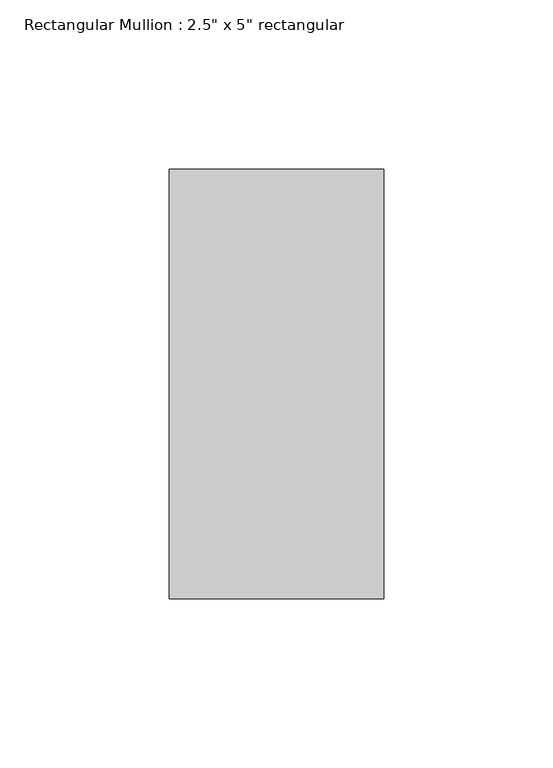
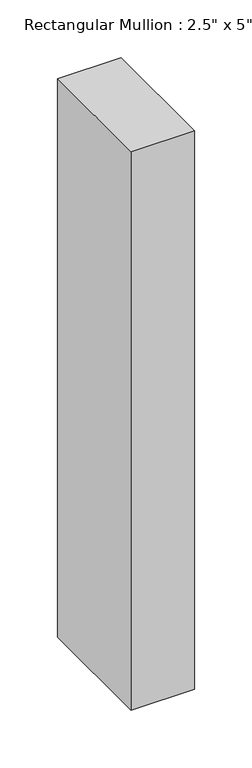
"""IFC4 building model written with IfcOpenShell, lengths in millimetres: member geometry."""

from ifc_helpers import new_model, si_unit, frame, origin, place, context, project, spatial, polyline, outline, extrude, source, transform, mapped, element, save


def member_e5d39754(model_context):
    return source(origin(), model_context, "Body", "SweptSolid", [
        extrude(outline(polyline([(0.0, 63.5), (0.0, -63.5), (-63.5, -63.5), (-63.5, 63.5), (0.0, 63.5)])), frame((0.0, 0.0, -590.55), z_axis=(0.0, 0.0, 1.0), x_axis=(1.0, 0.0, 0.0)), (0.0, 0.0, 1.0), 590.55),
    ])


if __name__ == "__main__":
    model = new_model("IFC4")
    model_context = context("Model", 3, world=origin())
    ifc_project = project(units=[si_unit("LENGTHUNIT", "METRE", prefix="MILLI")], contexts=[model_context])
    site = spatial("IfcSite", under=ifc_project)
    building = spatial("IfcBuilding", under=site)
    placement = place(None, origin())
    member_shape = member_e5d39754(model_context)
    element("IfcMember", 1, ObjectType="Rectangular Mullion : 2.5\" x 5\" rectangular", at=placement, inside=building, context=model_context, shape_type="MappedRepresentation", body=[
        mapped(member_shape, transform((0.0, 0.0, 0.0), x_axis=(1.0, 0.0, 0.0), y_axis=(0.0, 1.0, 0.0), z_axis=(0.0, 0.0, 1.0))),
    ])
    save(model, "model.ifc")

# Revit data of these elements
# Type "Rectangular Mullion : 2.5\" x 5\" rectangular"
#   built-in parameter 1007304 = 0.416667 (stored number, unit not read)
#   built-in parameter 1007301 = 0.104167 (stored number, unit not read)
#   built-in parameter 1007300 = 0.104167 (stored number, unit not read)
